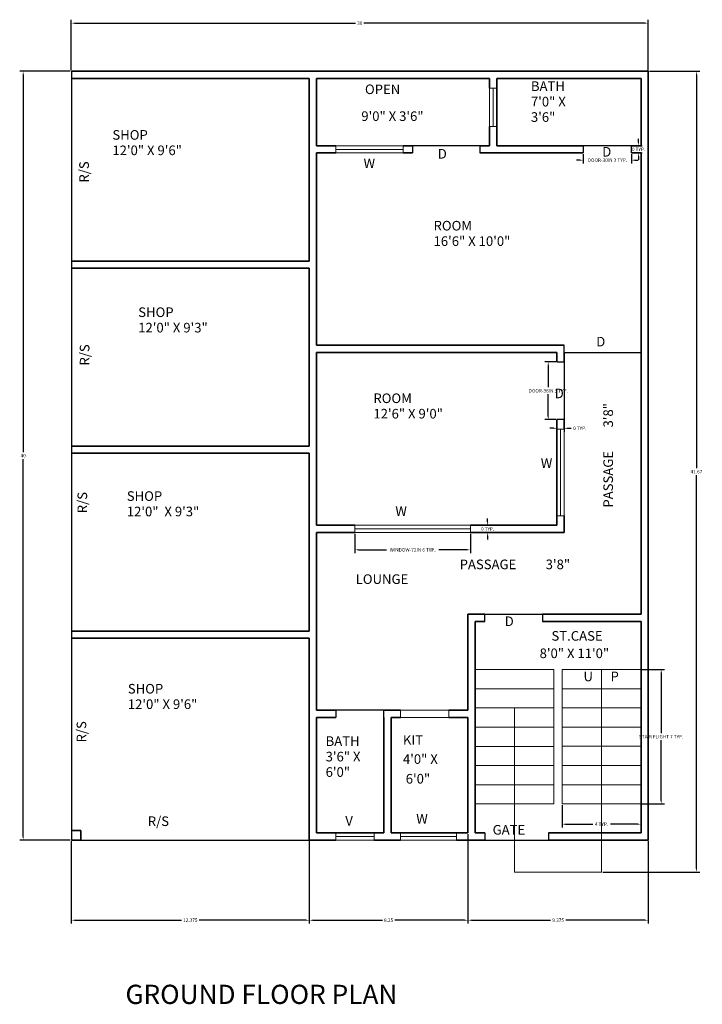
# Model space of a CAD drawing. Units: feet. Extents: x 60.2 to 151.6, y 170.7 to 222.6.
# Tile 1 of 3: x 60.2 to 95.6, y 171.3 to 222.6. Entities that reach past the tile are written whole.
import ezdxf

# ---------------------------------------------------------------- set-up
doc = ezdxf.new("R2010")
doc.units = ezdxf.units.FT
for name, color, linetype, lineweight in [('A-ANNO-DIMS', 7, 'Continuous', 13), ('A-ANNO-TEXT', 7, 'Continuous', 13), ('A-ANNO-TITL', 7, 'Continuous', 25), ('A-AREA-IDEN', 7, 'Continuous', 18), ('A-DOOR', 6, 'Continuous', 25), ('A-FLOR-STRS', 6, 'Continuous', 18), ('A-GLAZ', 240, 'Continuous', 18), ('A-WALL', 175, 'Continuous', 35)]:
    doc.layers.add(name, color=color, linetype=linetype, lineweight=lineweight)
doc.styles.get("Standard").update_dxf_attribs({"font": 'arial.ttf'})
doc.dimstyles.get("Standard").update_dxf_attribs({"dimtxt": 0.18, "dimasz": 0.18, "dimexe": 0.18, "dimexo": 0.0625, "dimgap": 0.09, "dimtad": 0, "dimtih": 1, "dimtoh": 1, "dimdec": 4, "dimzin": 0, "dimdsep": 46, "dimtxsty": 'Standard', "dimcen": 0.09, "dimadec": 0, "dimazin": 0, "dimtfac": 1, "dimtdec": 4, "dimtofl": 0, "dimtmove": 0, "dimatfit": 3, "dimfxl": 1, "dimtolj": 1, "dimtzin": 0, "dimarcsym": 0})

# ---------------------------------------------------------------- blocks, each defined once
blk = doc.blocks.new('DOOR-30IN')
for p, q in [((2.5, 0.375), (0, 0.375)), ((0, 0.375), (0, 0)), ((2.5, 0), (2.5, 0.375))]:
    blk.add_line(p, q)
blk = doc.blocks.new('DOOR-36IN')
for p, q in [((0, 0.375), (3, 0.375)), ((0, 0), (0, 0.375)), ((3, 0.375), (3, 0))]:
    blk.add_line(p, q)
blk = doc.blocks.new('DOOR-42IN')
for p, q in [((3.5, 0.375), (0, 0.375)), ((0, 0.375), (0, 0)), ((3.5, 0.375), (3.5, 0))]:
    blk.add_line(p, q)
blk = doc.blocks.new('WINDOW-24IN')
for p, q in [((0, 2), (0.375, 2)), ((0, 2), (0, 0)), ((0.188, 2), (0.188, 0)), ((0.375, 2), (0.375, 0)), ((0, 0), (0.375, 0))]:
    blk.add_line(p, q)
blk = doc.blocks.new('STAIR-FLIGHT-8-TREADS')
for p, q in [((0, 7), (4.1, 7)), ((4.1, 7), (4.1, 0)), ((0, 6), (4.1, 6)), ((0, 5), (4.1, 5)), ((0, 4), (4.1, 4)), ((0, 3), (4.1, 3)), ((0, 2), (4.1, 2)), ((0, 1), (4.1, 1)), ((0, 0), (4.1, 0))]:
    blk.add_line(p, q)
blk = doc.blocks.new('SHOP-BAY-WALL-12FT-X-9FT3IN')
for p, q in [((0.375, 9.25), (0, 9.25)), ((12.375, 9.25), (0.375, 9.25)), ((0.375, 9.25), (12.375, 9.25)), ((12.375, 9.25), (12.375, 0)), ((0.375, 0), (0, 0)), ((12.375, 0), (0.375, 0))]:
    blk.add_line(p, q)
blk = doc.blocks.new('WINDOW-72IN')
for p, q in [((0, 0.375), (0, 0)), ((6, 0.375), (0, 0.375)), ((0, 0.188), (6, 0.188)), ((6, 0), (0, 0)), ((6, 0), (6, 0.375))]:
    blk.add_line(p, q)
blk = doc.blocks.new('*D14')
at = {"layer": 'A-ANNO-DIMS', "color": 0, "lineweight": -2, "transparency": 16777216}
for p, q in [((89.282, 215.268), (89.102, 215.268)), ((89.462, 215.581), (89.462, 215.088)), ((91.962, 215.581), (91.962, 215.088)), ((92.142, 215.268), (92.322, 215.268))]:
    blk.add_line(p, q, dxfattribs=at)
at = {"layer": 'A-ANNO-DIMS', "color": 0, "transparency": 16777216}
for points in [[(89.282, 215.298), (89.282, 215.238), (89.462, 215.268)], [(92.142, 215.298), (92.142, 215.238), (91.962, 215.268)]]:
    blk.add_solid(points, dxfattribs=at)
at = {"layer": 'Defpoints', "color": 0, "transparency": 16777216}
for p in [(89.462, 215.643), (91.962, 215.643), (91.962, 215.268)]:
    blk.add_point(p, dxfattribs=at)
at = {"layer": 'A-ANNO-DIMS', "color": 0, "transparency": 16777216, "insert": (90.712, 215.268), "char_height": 0.18, "attachment_point": 5}
blk.add_mtext('\\A1;DOOR-30IN 3 TYP.', dxfattribs=at)
blk = doc.blocks.new('*D15')
at = {"layer": 'A-ANNO-DIMS', "color": 0, "lineweight": -2, "transparency": 16777216}
for p, q in [((92.337, 216.198), (92.337, 216.378)), ((92.025, 216.018), (92.517, 216.018)), ((92.025, 215.643), (92.517, 215.643)), ((92.337, 215.463), (92.337, 215.283))]:
    blk.add_line(p, q, dxfattribs=at)
at = {"layer": 'A-ANNO-DIMS', "color": 0, "transparency": 16777216}
for points in [[(92.307, 216.198), (92.367, 216.198), (92.337, 216.018)], [(92.307, 215.463), (92.367, 215.463), (92.337, 215.643)]]:
    blk.add_solid(points, dxfattribs=at)
at = {"layer": 'Defpoints', "color": 0, "transparency": 16777216}
for p in [(91.962, 216.018), (92.337, 216.018), (91.962, 215.643)]:
    blk.add_point(p, dxfattribs=at)
at = {"layer": 'A-ANNO-DIMS', "color": 0, "transparency": 16777216, "insert": (92.337, 215.831), "char_height": 0.18, "attachment_point": 5}
blk.add_mtext('\\A1;0 TYP.', dxfattribs=at)
blk = doc.blocks.new('*D16')
at = {"layer": 'A-ANNO-DIMS', "color": 0, "lineweight": -2, "transparency": 16777216}
for p, q in [((88.025, 204.768), (87.457, 204.768)), ((87.637, 204.588), (87.637, 203.451)), ((87.637, 201.948), (87.637, 203.085)), ((88.025, 201.768), (87.457, 201.768))]:
    blk.add_line(p, q, dxfattribs=at)
at = {"layer": 'A-ANNO-DIMS', "color": 0, "transparency": 16777216}
for points in [[(87.607, 204.588), (87.667, 204.588), (87.637, 204.768)], [(87.607, 201.948), (87.667, 201.948), (87.637, 201.768)]]:
    blk.add_solid(points, dxfattribs=at)
at = {"layer": 'Defpoints', "color": 0, "transparency": 16777216}
for p in [(88.087, 204.768), (87.637, 201.768), (88.087, 201.768)]:
    blk.add_point(p, dxfattribs=at)
at = {"layer": 'A-ANNO-DIMS', "color": 0, "transparency": 16777216, "insert": (87.637, 203.268), "char_height": 0.18, "attachment_point": 5}
blk.add_mtext('\\A1;DOOR-36IN 3 TYP.', dxfattribs=at)
blk = doc.blocks.new('*D17')
at = {"layer": 'A-ANNO-DIMS', "color": 0, "lineweight": -2, "transparency": 16777216}
for p, q in [((88.087, 201.706), (88.087, 201.138)), ((88.462, 201.706), (88.462, 201.138)), ((87.907, 201.318), (87.727, 201.318)), ((88.642, 201.318), (88.822, 201.318))]:
    blk.add_line(p, q, dxfattribs=at)
at = {"layer": 'A-ANNO-DIMS', "color": 0, "transparency": 16777216}
for points in [[(87.907, 201.348), (87.907, 201.288), (88.087, 201.318)], [(88.642, 201.348), (88.642, 201.288), (88.462, 201.318)]]:
    blk.add_solid(points, dxfattribs=at)
at = {"layer": 'Defpoints', "color": 0, "transparency": 16777216}
for p in [(88.087, 201.768), (88.462, 201.768), (88.462, 201.318)]:
    blk.add_point(p, dxfattribs=at)
at = {"layer": 'A-ANNO-DIMS', "color": 0, "transparency": 16777216, "insert": (89.28, 201.318), "char_height": 0.18, "attachment_point": 5}
blk.add_mtext('\\A1;0 TYP.', dxfattribs=at)
blk = doc.blocks.new('*D32')
at = {"layer": 'A-ANNO-DIMS', "color": 0, "lineweight": -2, "transparency": 16777216}
for p, q in [((77.587, 195.831), (77.587, 194.813)), ((83.587, 195.831), (83.587, 194.813)), ((77.767, 194.993), (79.231, 194.993)), ((83.407, 194.993), (81.943, 194.993))]:
    blk.add_line(p, q, dxfattribs=at)
at = {"layer": 'A-ANNO-DIMS', "color": 0, "transparency": 16777216}
for points in [[(77.767, 195.023), (77.767, 194.963), (77.587, 194.993)], [(83.407, 195.023), (83.407, 194.963), (83.587, 194.993)]]:
    blk.add_solid(points, dxfattribs=at)
at = {"layer": 'Defpoints', "color": 0, "transparency": 16777216}
for p in [(77.587, 195.893), (83.587, 195.893), (83.587, 194.993)]:
    blk.add_point(p, dxfattribs=at)
at = {"layer": 'A-ANNO-DIMS', "color": 0, "transparency": 16777216, "insert": (80.587, 194.993), "char_height": 0.18, "attachment_point": 5}
blk.add_mtext('\\A1;WINDOW-72IN 6 TYP.', dxfattribs=at)
blk = doc.blocks.new('*D33')
at = {"layer": 'A-ANNO-DIMS', "color": 0, "lineweight": -2, "transparency": 16777216}
for p, q in [((83.65, 196.268), (84.667, 196.268)), ((84.487, 196.448), (84.487, 196.628)), ((83.65, 195.893), (84.667, 195.893)), ((84.487, 195.713), (84.487, 195.533))]:
    blk.add_line(p, q, dxfattribs=at)
at = {"layer": 'A-ANNO-DIMS', "color": 0, "transparency": 16777216}
for points in [[(84.457, 196.448), (84.517, 196.448), (84.487, 196.268)], [(84.457, 195.713), (84.517, 195.713), (84.487, 195.893)]]:
    blk.add_solid(points, dxfattribs=at)
at = {"layer": 'Defpoints', "color": 0, "transparency": 16777216}
for p in [(83.587, 196.268), (84.487, 196.268), (83.587, 195.893)]:
    blk.add_point(p, dxfattribs=at)
at = {"layer": 'A-ANNO-DIMS', "color": 0, "transparency": 16777216, "insert": (84.487, 196.081), "char_height": 0.18, "attachment_point": 5}
blk.add_mtext('\\A1;0 TYP.', dxfattribs=at)
blk = doc.blocks.new('*D34')
at = {"layer": 'A-ANNO-DIMS', "color": 0, "lineweight": -2, "transparency": 16777216}
for p, q in [((92.525, 188.768), (93.692, 188.768)), ((93.512, 188.588), (93.512, 185.451)), ((93.512, 181.948), (93.512, 185.085)), ((92.525, 181.768), (93.692, 181.768))]:
    blk.add_line(p, q, dxfattribs=at)
at = {"layer": 'A-ANNO-DIMS', "color": 0, "transparency": 16777216}
for points in [[(93.482, 188.588), (93.542, 188.588), (93.512, 188.768)], [(93.482, 181.948), (93.542, 181.948), (93.512, 181.768)]]:
    blk.add_solid(points, dxfattribs=at)
at = {"layer": 'Defpoints', "color": 0, "transparency": 16777216}
for p in [(92.462, 188.768), (92.462, 181.768), (93.512, 181.768)]:
    blk.add_point(p, dxfattribs=at)
at = {"layer": 'A-ANNO-DIMS', "color": 0, "transparency": 16777216, "insert": (93.512, 185.268), "char_height": 0.18, "attachment_point": 5}
blk.add_mtext('\\A1;STAIR FLIGHT 7 TYP.', dxfattribs=at)
blk = doc.blocks.new('*D35')
at = {"layer": 'A-ANNO-DIMS', "color": 0, "lineweight": -2, "transparency": 16777216}
for p, q in [((88.362, 181.706), (88.362, 180.538)), ((92.462, 181.706), (92.462, 180.538)), ((88.542, 180.718), (89.95, 180.718)), ((92.282, 180.718), (90.874, 180.718))]:
    blk.add_line(p, q, dxfattribs=at)
at = {"layer": 'A-ANNO-DIMS', "color": 0, "transparency": 16777216}
for points in [[(88.542, 180.748), (88.542, 180.688), (88.362, 180.718)], [(92.282, 180.748), (92.282, 180.688), (92.462, 180.718)]]:
    blk.add_solid(points, dxfattribs=at)
at = {"layer": 'Defpoints', "color": 0, "transparency": 16777216}
for p in [(88.362, 181.768), (92.462, 181.768), (88.362, 180.718)]:
    blk.add_point(p, dxfattribs=at)
at = {"layer": 'A-ANNO-DIMS', "color": 0, "transparency": 16777216, "insert": (90.412, 180.718), "char_height": 0.18, "attachment_point": 5}
blk.add_mtext('\\A1;4 TYP.', dxfattribs=at)
blk = doc.blocks.new('*D38')
at = {"layer": 'A-ANNO-DIMS', "color": 0, "lineweight": -2, "transparency": 16777216}
for p, q in [((62.837, 219.956), (62.837, 222.578)), ((63.017, 222.398), (77.619, 222.398)), ((92.657, 222.398), (78.056, 222.398)), ((92.837, 219.956), (92.837, 222.578))]:
    blk.add_line(p, q, dxfattribs=at)
at = {"layer": 'A-ANNO-DIMS', "color": 0, "transparency": 16777216}
for points in [[(63.017, 222.428), (63.017, 222.368), (62.837, 222.398)], [(92.657, 222.428), (92.657, 222.368), (92.837, 222.398)]]:
    blk.add_solid(points, dxfattribs=at)
at = {"layer": 'Defpoints', "color": 0, "transparency": 16777216}
for p in [(92.837, 222.398), (62.837, 219.893), (92.837, 219.893)]:
    blk.add_point(p, dxfattribs=at)
at = {"layer": 'A-ANNO-DIMS', "color": 0, "transparency": 16777216, "insert": (77.837, 222.398), "char_height": 0.18, "attachment_point": 5}
blk.add_mtext('\\A1;30', dxfattribs=at)
blk = doc.blocks.new('*D39')
at = {"layer": 'A-ANNO-DIMS', "color": 0, "lineweight": -2, "transparency": 16777216}
for p, q in [((92.9, 219.893), (95.522, 219.893)), ((95.342, 219.713), (95.342, 199.242)), ((95.342, 178.406), (95.342, 198.878)), ((90.475, 178.226), (95.522, 178.226))]:
    blk.add_line(p, q, dxfattribs=at)
at = {"layer": 'A-ANNO-DIMS', "color": 0, "transparency": 16777216}
for points in [[(95.312, 219.713), (95.372, 219.713), (95.342, 219.893)], [(95.312, 178.406), (95.372, 178.406), (95.342, 178.226)]]:
    blk.add_solid(points, dxfattribs=at)
at = {"layer": 'Defpoints', "color": 0, "transparency": 16777216}
for p in [(92.837, 219.893), (95.342, 219.893), (90.412, 178.226)]:
    blk.add_point(p, dxfattribs=at)
at = {"layer": 'A-ANNO-DIMS', "color": 0, "transparency": 16777216, "insert": (95.342, 199.06), "char_height": 0.18, "attachment_point": 5}
blk.add_mtext('\\A1;41.67', dxfattribs=at)
blk = doc.blocks.new('*D40')
at = {"layer": 'A-ANNO-DIMS', "color": 0, "lineweight": -2, "transparency": 16777216}
for p, q in [((62.775, 219.893), (60.152, 219.893)), ((60.332, 219.713), (60.332, 200.075)), ((60.332, 180.073), (60.332, 199.711)), ((62.775, 179.893), (60.152, 179.893))]:
    blk.add_line(p, q, dxfattribs=at)
at = {"layer": 'A-ANNO-DIMS', "color": 0, "transparency": 16777216}
for points in [[(60.302, 219.713), (60.362, 219.713), (60.332, 219.893)], [(60.302, 180.073), (60.362, 180.073), (60.332, 179.893)]]:
    blk.add_solid(points, dxfattribs=at)
at = {"layer": 'Defpoints', "color": 0, "transparency": 16777216}
for p in [(60.332, 219.893), (62.837, 219.893), (62.837, 179.893)]:
    blk.add_point(p, dxfattribs=at)
at = {"layer": 'A-ANNO-DIMS', "color": 0, "transparency": 16777216, "insert": (60.332, 199.893), "char_height": 0.18, "attachment_point": 5}
blk.add_mtext('\\A1;40', dxfattribs=at)
blk = doc.blocks.new('*D41')
at = {"layer": 'A-ANNO-DIMS', "color": 0, "lineweight": -2, "transparency": 16777216}
for p, q in [((62.837, 179.831), (62.837, 175.541)), ((75.212, 179.831), (75.212, 175.541)), ((63.017, 175.721), (68.569, 175.721)), ((75.032, 175.721), (69.481, 175.721))]:
    blk.add_line(p, q, dxfattribs=at)
at = {"layer": 'A-ANNO-DIMS', "color": 0, "transparency": 16777216}
for points in [[(63.017, 175.751), (63.017, 175.691), (62.837, 175.721)], [(75.032, 175.751), (75.032, 175.691), (75.212, 175.721)]]:
    blk.add_solid(points, dxfattribs=at)
at = {"layer": 'Defpoints', "color": 0, "transparency": 16777216}
for p in [(62.837, 179.893), (75.212, 179.893), (75.212, 175.721)]:
    blk.add_point(p, dxfattribs=at)
at = {"layer": 'A-ANNO-DIMS', "color": 0, "transparency": 16777216, "insert": (69.025, 175.721), "char_height": 0.18, "attachment_point": 5}
blk.add_mtext('\\A1;12.375', dxfattribs=at)
blk = doc.blocks.new('*D42')
at = {"layer": 'A-ANNO-DIMS', "color": 0, "lineweight": -2, "transparency": 16777216}
for p, q in [((75.212, 179.831), (75.212, 175.541)), ((83.462, 180.206), (83.462, 175.541)), ((75.392, 175.721), (79.013, 175.721)), ((83.282, 175.721), (79.662, 175.721))]:
    blk.add_line(p, q, dxfattribs=at)
at = {"layer": 'A-ANNO-DIMS', "color": 0, "transparency": 16777216}
for points in [[(75.392, 175.751), (75.392, 175.691), (75.212, 175.721)], [(83.282, 175.751), (83.282, 175.691), (83.462, 175.721)]]:
    blk.add_solid(points, dxfattribs=at)
at = {"layer": 'Defpoints', "color": 0, "transparency": 16777216}
for p in [(75.212, 179.893), (83.462, 180.268), (83.462, 175.721)]:
    blk.add_point(p, dxfattribs=at)
at = {"layer": 'A-ANNO-DIMS', "color": 0, "transparency": 16777216, "insert": (79.337, 175.721), "char_height": 0.18, "attachment_point": 5}
blk.add_mtext('\\A1;8.25', dxfattribs=at)
blk = doc.blocks.new('*D43')
at = {"layer": 'A-ANNO-DIMS', "color": 0, "lineweight": -2, "transparency": 16777216}
for p, q in [((83.462, 180.206), (83.462, 175.541)), ((92.837, 179.831), (92.837, 175.541)), ((83.642, 175.721), (87.755, 175.721)), ((92.657, 175.721), (88.544, 175.721))]:
    blk.add_line(p, q, dxfattribs=at)
at = {"layer": 'A-ANNO-DIMS', "color": 0, "transparency": 16777216}
for points in [[(83.642, 175.751), (83.642, 175.691), (83.462, 175.721)], [(92.657, 175.751), (92.657, 175.691), (92.837, 175.721)]]:
    blk.add_solid(points, dxfattribs=at)
at = {"layer": 'Defpoints', "color": 0, "transparency": 16777216}
for p in [(83.462, 180.268), (92.837, 179.893), (92.837, 175.721)]:
    blk.add_point(p, dxfattribs=at)
at = {"layer": 'A-ANNO-DIMS', "color": 0, "transparency": 16777216, "insert": (88.15, 175.721), "char_height": 0.18, "attachment_point": 5}
blk.add_mtext('\\A1;9.375', dxfattribs=at)

msp = doc.modelspace()

# ---------------------------------------------------------------- linework, layer by layer
at = {"layer": 'A-DOOR'}
for p, q in [((88.4623, 205.2682), (88.4623, 205.6432)), ((88.4623, 205.2682), (92.4623, 205.2682)), ((84.3373, 180.2682), (84.3373, 179.8932)), ((87.6498, 180.2682), (87.6498, 179.8932))]:
    msp.add_line(p, q, dxfattribs=at)
for points in [[(62.8373, 219.8932), (62.8373, 179.8932)], [(62.8373, 179.8932), (75.2123, 179.8932)], [(84.3373, 179.8932), (87.6498, 179.8932)]]:
    msp.add_lwpolyline(points, dxfattribs=at)
at = {"layer": 'A-FLOR-STRS'}
for p, q in [((90.4123, 178.2264), (90.4123, 188.7682)), ((85.8873, 186.7682), (85.8873, 178.2264)), ((85.8873, 178.2264), (90.4123, 178.2264))]:
    msp.add_line(p, q, dxfattribs=at)
at = {"layer": 'A-GLAZ'}
for p, q in [((76.5873, 216.0182), (76.5873, 215.6432)), ((80.0873, 216.0182), (76.5873, 216.0182)), ((76.5873, 215.8307), (80.0873, 215.8307)), ((80.0873, 215.6432), (80.0873, 216.0182)), ((80.0873, 215.6432), (76.5873, 215.6432)), ((88.0873, 200.7682), (88.0873, 201.2682)), ((88.0873, 201.2682), (88.4623, 201.2682)), ((88.2748, 201.2682), (88.2748, 196.7682)), ((88.4623, 201.2682), (88.4623, 196.7682)), ((88.0873, 196.7682), (88.0873, 200.7682)), ((88.0873, 196.7682), (88.4623, 196.7682)), ((77.5873, 195.8932), (81.5873, 195.8932)), ((81.5873, 195.8932), (82.5873, 195.8932)), ((82.5873, 195.8932), (83.5873, 195.8932)), ((79.9623, 186.2682), (79.9623, 186.6432)), ((82.4623, 186.6432), (79.9623, 186.6432)), ((82.4623, 186.6432), (82.4623, 186.2682)), ((82.4623, 186.2682), (79.9623, 186.2682)), ((76.5873, 180.2682), (76.5873, 179.8932)), ((76.5873, 180.2682), (78.5873, 180.2682)), ((76.5873, 180.0807), (78.5873, 180.0807)), ((78.5873, 180.2682), (78.5873, 179.8932)), ((79.9623, 180.2682), (79.9623, 179.8932)), ((79.9623, 180.2682), (82.8623, 180.2682)), ((79.9623, 180.0807), (82.8623, 180.0807)), ((82.8623, 180.2682), (82.8623, 179.8932))]:
    msp.add_line(p, q, dxfattribs=at)
for points in [[(76.5873, 179.8932), (78.5873, 179.8932)], [(79.9623, 179.8932), (82.8623, 179.8932)]]:
    msp.add_lwpolyline(points, dxfattribs=at)
at = {"layer": 'A-WALL'}
for p, q in [((63.2123, 219.5182), (62.8373, 219.5182)), ((63.2123, 219.5182), (75.2123, 219.5182)), ((75.2123, 219.5182), (75.2123, 210.0182)), ((75.5873, 219.5182), (75.5873, 216.0182)), ((75.5873, 219.5182), (84.5873, 219.5182)), ((84.5873, 219.5182), (84.5873, 219.0182)), ((84.5873, 219.5182), (84.5873, 219.0182)), ((84.9623, 219.5182), (84.9623, 216.0182)), ((84.9623, 219.5182), (84.9623, 219.0182)), ((84.5873, 216.0182), (84.5873, 217.0182)), ((84.5873, 217.0182), (84.5873, 216.0182)), ((84.9623, 217.0182), (84.9623, 216.0182)), ((75.5873, 216.0182), (76.5873, 216.0182)), ((76.5873, 216.0182), (75.5873, 216.0182)), ((80.0873, 216.0182), (80.5873, 216.0182)), ((80.5873, 216.0182), (80.0873, 216.0182)), ((84.5873, 216.0182), (84.0873, 216.0182)), ((84.5873, 216.0182), (84.0873, 216.0182)), ((84.9623, 216.0182), (89.4623, 216.0182)), ((84.9623, 216.0182), (88.4623, 216.0182)), ((88.4623, 216.0182), (89.4623, 216.0182)), ((91.9623, 216.0182), (92.4623, 216.0182)), ((92.4623, 216.0182), (91.9623, 216.0182)), ((75.5873, 215.6432), (75.5873, 205.6432)), ((75.5873, 215.6432), (75.5873, 210.0182)), ((76.5873, 215.6432), (75.5873, 215.6432)), ((80.5873, 215.6432), (80.0873, 215.6432)), ((80.5873, 215.6432), (80.0873, 215.6432)), ((84.0873, 215.6432), (84.9623, 215.6432)), ((84.9623, 215.6432), (89.4623, 215.6432)), ((91.9623, 215.6432), (92.4623, 215.6432)), ((63.2123, 210.0182), (62.8373, 210.0182)), ((75.2123, 210.0182), (63.2123, 210.0182)), ((75.5873, 209.6432), (75.5873, 205.6432)), ((75.5873, 205.6432), (88.4623, 205.6432)), ((75.5873, 205.2682), (88.0873, 205.2682)), ((75.5873, 205.2682), (88.0873, 205.2682)), ((75.5873, 205.2682), (75.5873, 200.3932)), ((88.0873, 205.2682), (88.0873, 204.7682)), ((88.0873, 205.2682), (88.0873, 204.7682)), ((88.4623, 205.2682), (88.4623, 204.7682)), ((88.0873, 201.2682), (88.0873, 201.7682)), ((88.0873, 201.7682), (88.0873, 196.2682)), ((88.4623, 201.7682), (88.4623, 201.2682)), ((75.5873, 200.3932), (75.5873, 200.0182)), ((75.5873, 200.0182), (75.5873, 196.2682)), ((88.0873, 196.2682), (88.0873, 196.7682)), ((88.0873, 196.2682), (88.0873, 196.7682)), ((88.4623, 196.7682), (88.4623, 196.2682)), ((75.5873, 196.2682), (77.5873, 196.2682)), ((77.5873, 196.2682), (75.5873, 196.2682)), ((88.0873, 196.2682), (83.5873, 196.2682)), ((88.4623, 196.2682), (88.4623, 195.8932)), ((75.5873, 195.8932), (75.5873, 190.7682)), ((77.5873, 195.8932), (75.5873, 195.8932)), ((88.0873, 195.8932), (83.5873, 195.8932)), ((88.4623, 195.8932), (88.0873, 195.8932)), ((83.8373, 191.6432), (83.4623, 191.6432)), ((83.4623, 191.6432), (83.4623, 191.2682)), ((83.8373, 191.6432), (84.3373, 191.6432)), ((87.8373, 191.6432), (87.3373, 191.6432)), ((87.3373, 191.6432), (91.8373, 191.6432)), ((92.4623, 191.6432), (87.8373, 191.6432)), ((91.8373, 191.6432), (92.4623, 191.6432)), ((83.4623, 186.6432), (83.4623, 191.2682)), ((83.8373, 180.2682), (83.8373, 191.2682)), ((83.8373, 191.2682), (84.3373, 191.2682)), ((83.8373, 191.2682), (84.3373, 191.2682)), ((87.3373, 191.2682), (91.8373, 191.2682)), ((91.8373, 191.2682), (92.4623, 191.2682)), ((75.5873, 190.7682), (75.5873, 190.3932)), ((63.2123, 190.3932), (62.8373, 190.3932)), ((75.2123, 190.3932), (63.2123, 190.3932)), ((63.2123, 190.3932), (75.2123, 190.3932)), ((75.2123, 190.3932), (75.2123, 179.8932)), ((75.5873, 190.3932), (75.5873, 186.6432)), ((75.5873, 186.6432), (76.5873, 186.6432)), ((76.5873, 186.6432), (75.5873, 186.6432)), ((79.0873, 186.6432), (79.4623, 186.6432)), ((79.9623, 186.6432), (79.4623, 186.6432)), ((83.4623, 186.6432), (82.4623, 186.6432)), ((82.9623, 186.6432), (82.4623, 186.6432)), ((83.4623, 186.6432), (82.9623, 186.6432)), ((76.5873, 186.2682), (75.5873, 186.2682)), ((75.5873, 186.2682), (75.5873, 180.2682)), ((79.0873, 180.2682), (79.0873, 186.2682)), ((79.4623, 180.2682), (79.4623, 186.2682)), ((79.4623, 186.2682), (79.9623, 186.2682)), ((79.9623, 186.2682), (79.4623, 186.2682)), ((83.4623, 186.2682), (82.4623, 186.2682)), ((83.4623, 180.2682), (83.4623, 186.2682)), ((83.4623, 180.2682), (83.4623, 186.2682)), ((83.8373, 180.2682), (83.8373, 186.2682)), ((63.3373, 180.3932), (62.8373, 180.3932)), ((63.3373, 179.8932), (63.3373, 180.3932)), ((62.8373, 179.8932), (63.3373, 179.8932)), ((75.5873, 180.2682), (76.5873, 180.2682)), ((75.5873, 180.2682), (76.5873, 180.2682)), ((79.0873, 180.2682), (78.5873, 180.2682)), ((78.5873, 180.2682), (79.0873, 180.2682)), ((79.4623, 180.2682), (79.9623, 180.2682)), ((79.4623, 180.2682), (79.9623, 180.2682)), ((83.4623, 180.2682), (82.8623, 180.2682)), ((82.8623, 180.2682), (83.4623, 180.2682)), ((83.8373, 180.2682), (84.3373, 180.2682)), ((88.1498, 180.2682), (87.6498, 180.2682)), ((92.4623, 180.2682), (88.1498, 180.2682))]:
    msp.add_line(p, q, dxfattribs=at)
for points in [[(87.6498, 179.8932), (92.8373, 179.8932), (92.8373, 219.8932), (62.8373, 219.8932)], [(75.2123, 219.5182), (63.2123, 219.5182)], [(84.5873, 219.5182), (75.5873, 219.5182)], [(92.4623, 216.0182), (92.4623, 219.5182), (84.9623, 219.5182)], [(92.4623, 191.6432), (92.4623, 215.6432)], [(87.6498, 180.2682), (92.4623, 180.2682), (92.4623, 191.2682)], [(75.2123, 179.8932), (76.5873, 179.8932)], [(75.5873, 180.2682), (79.0873, 180.2682)], [(78.5873, 179.8932), (79.9623, 179.8932)], [(79.4623, 180.2682), (83.4623, 180.2682)], [(82.8623, 179.8932), (84.3373, 179.8932)], [(83.8373, 180.2682), (84.3373, 180.2682)]]:
    msp.add_lwpolyline(points, dxfattribs=at)

# ---------------------------------------------------------------- block references
at = {"layer": 'A-DOOR'}
for name, p in [('DOOR-42IN', (80.587, 215.643)), ('DOOR-30IN', (89.462, 215.643)), ('DOOR-36IN', (84.337, 191.268)), ('DOOR-30IN', (76.587, 186.268))]:
    msp.add_blockref(name, p, dxfattribs=at)
at = {"layer": 'A-DOOR', "rotation": 269.9999999999999}
msp.add_blockref('DOOR-36IN', (88.0871, 204.7685), dxfattribs=at)
at = {"layer": 'A-FLOR-STRS'}
msp.add_blockref('STAIR-FLIGHT-8-TREADS', (83.837, 181.768), dxfattribs=at)
at = {"layer": 'A-FLOR-STRS', "rotation": 180}
msp.add_blockref('STAIR-FLIGHT-8-TREADS', (92.4625, 188.7684), dxfattribs=at)
at = {"layer": 'A-GLAZ'}
for name, p in [('WINDOW-24IN', (84.587, 217.018)), ('WINDOW-72IN', (77.587, 195.893))]:
    msp.add_blockref(name, p, dxfattribs=at)
at = {"layer": 'A-WALL'}
for p in [(62.837, 200.393), (62.837, 190.768)]:
    msp.add_blockref('SHOP-BAY-WALL-12FT-X-9FT3IN', p, dxfattribs=at)

# ---------------------------------------------------------------- texts
at = {"layer": 'A-ANNO-DIMS'}
for s, p in [('7\'0" X', (86.7368, 218.0655)), ('9\'0" X 3\'6"', (77.9166, 217.3088)), ('3\'6"', (86.7368, 217.2623)), ('12\'0" X 9\'6"', (64.9716, 215.5299)), ('16\'6" X 10\'0"', (81.6736, 210.8062)), ('12\'0" X 9\'3"', (66.3156, 206.3046)), ('12\'6" X 9\'0"', (78.5449, 201.8268)), ('12\'0"  X 9\'3"', (65.7221, 196.7377)), ('8\'0" X 11\'0"', (87.1894, 189.3586)), ('12\'0" X 9\'6"', (65.7757, 186.7114)), ('3\'6" X', (76.0609, 183.9841)), ('4\'0" X', (80.0809, 183.8552)), ('6\'0"', (76.0609, 183.1809)), ('6\'0"', (80.2272, 182.832))]:
    msp.add_text(s, height=0.5, dxfattribs=at).set_placement(p)
at = {"layer": 'A-ANNO-TEXT'}
for s, p in [('D', (81.8958, 215.3501)), ('D', (90.4471, 215.4551)), ('W', (78.0337, 214.8531)), ('D', (90.1352, 205.5758)), ('D', (87.9747, 202.8813)), ('W', (87.2502, 199.252)), ('W', (79.6882, 196.7573)), ('D', (85.3753, 191.0249)), ('U', (89.4714, 188.1567)), ('P', (90.878, 188.1577)), ('R/S', (66.8125, 180.6218)), ('V', (77.0856, 180.6423)), ('W', (80.7745, 180.7447)), ('GATE', (84.7458, 180.1742))]:
    msp.add_text(s, height=0.5, dxfattribs=at).set_placement(p)
for p in [(63.7493, 214.1004), (63.7781, 204.5808), (63.658, 196.8949), (63.612, 184.9696)]:
    msp.add_text('R/S', height=0.5, rotation=90, dxfattribs=at).set_placement(p)
at = {"layer": 'A-ANNO-TITL'}
msp.add_text('GROUND FLOOR PLAN', height=1, dxfattribs=at).set_placement((65.6506, 171.3626))
at = {"layer": 'A-AREA-IDEN'}
for s, p in [('BATH', (86.7368, 218.8687)), ('OPEN', (78.1073, 218.7051)), ('SHOP', (64.9716, 216.3331)), ('ROOM', (81.6736, 211.6094)), ('SHOP', (66.3156, 207.1078)), ('ROOM', (78.5449, 202.63)), ('SHOP', (65.7221, 197.5409)), ('PASSAGE          3\'8"', (83.0301, 193.9861)), ('LOUNGE', (77.6249, 193.2182)), ('ST.CASE', (87.8038, 190.2648)), ('SHOP', (65.7757, 187.5146)), ('BATH', (76.0609, 184.7873)), ('KIT', (80.0809, 184.8492))]:
    msp.add_text(s, height=0.5, dxfattribs=at).set_placement(p)
msp.add_text('PASSAGE        3\'8"', height=0.5, rotation=90, dxfattribs=at).set_placement((91.0053, 197.1911))

# ---------------------------------------------------------------- dimensions: what is measured, and where the dimension line sits
at = {"layer": 'A-ANNO-DIMS'}
for base, p1, p2, override, picture, middle in [((92.8373, 222.3982), (62.8373, 219.8932), (92.8373, 219.8932), {"dimdec": 0, "dimlfac": 1, "dimrnd": 0, "dimzin": 0, "dimdsep": 46, "dimlunit": 2}, '*D38', (77.8373, 222.3982)), ((75.2123, 175.7214), (62.8373, 179.8932), (75.2123, 179.8932), {"dimdec": 3, "dimlfac": 1, "dimrnd": 0, "dimzin": 0, "dimdsep": 46, "dimlunit": 2}, '*D41', (69.0248, 175.7214)), ((83.4623, 175.7214), (75.2123, 179.8932), (83.4623, 180.2682), {"dimdec": 2, "dimlfac": 1, "dimrnd": 0, "dimzin": 0, "dimdsep": 46, "dimlunit": 2}, '*D42', (79.3373, 175.7214)), ((92.8373, 175.7214), (83.4623, 180.2682), (92.8373, 179.8932), {"dimdec": 3, "dimlfac": 1, "dimrnd": 0, "dimzin": 0, "dimdsep": 46, "dimlunit": 2}, '*D43', (88.1498, 175.7214))]:
    dim = msp.add_linear_dim(base=base, p1=p1, p2=p2, dimstyle='Standard', override=override, dxfattribs=at)
    dim.commit()
    dim.dimension.update_dxf_attribs({"geometry": picture, "text_midpoint": middle})
for base, p1, p2, override, picture, middle in [((60.3323, 219.8932), (62.8373, 179.8932), (62.8373, 219.8932), {"dimdec": 0, "dimlfac": 1, "dimrnd": 0, "dimzin": 0, "dimdsep": 46, "dimlunit": 2}, '*D40', (60.3323, 199.8932)), ((95.3423, 219.8932), (90.4123, 178.2264), (92.8373, 219.8932), {"dimdec": 2, "dimlfac": 1, "dimrnd": 0, "dimzin": 0, "dimdsep": 46, "dimlunit": 2}, '*D39', (95.3423, 199.0598))]:
    dim = msp.add_linear_dim(base=base, p1=p1, p2=p2, angle=90, dimstyle='Standard', override=override, dxfattribs=at)
    dim.commit()
    dim.dimension.update_dxf_attribs({"geometry": picture, "text_midpoint": middle})
for base, p1, p2, angle, text, picture, middle in [((92.3373, 216.0182), (91.9623, 215.6432), (91.9623, 216.0182), 90, '<> TYP.', '*D15', (92.3373, 215.8307)), ((87.6373, 201.7682), (88.0873, 204.7682), (88.0873, 201.7682), 270, 'DOOR-36IN <> TYP.', '*D16', (87.6373, 203.2682)), ((84.4873, 196.2682), (83.5873, 195.8932), (83.5873, 196.2682), 90, '<> TYP.', '*D33', (84.4873, 196.0807)), ((93.5123, 181.7682), (92.4623, 188.7682), (92.4623, 181.7682), 270, 'STAIR FLIGHT <> TYP.', '*D34', (93.5123, 185.2682)), ((88.3623, 180.7182), (92.4623, 181.7682), (88.3623, 181.7682), 180, '<> TYP.', '*D35', (90.4123, 180.7182))]:
    dim = msp.add_linear_dim(base=base, p1=p1, p2=p2, angle=angle, text=text, dimstyle='Standard', override={"dimdec": 0, "dimlfac": 1, "dimrnd": 0, "dimzin": 0, "dimdsep": 46, "dimlunit": 2}, dxfattribs=at)
    dim.commit()
    dim.dimension.update_dxf_attribs({"geometry": picture, "text_midpoint": middle})
for base, p1, p2, text, picture, middle in [((91.962252404, 215.2682003807), (89.462252404, 215.6432003807), (91.962252404, 215.6432003807), 'DOOR-30IN <> TYP.', '*D14', (90.712252404, 215.2682003807)), ((88.4623, 201.3182), (88.0873, 201.7682), (88.4623, 201.7682), '<> TYP.', '*D17', (89.2804, 201.3182)), ((83.5873, 194.9932), (77.5873, 195.8932), (83.5873, 195.8932), 'WINDOW-72IN <> TYP.', '*D32', (80.5873, 194.9932))]:
    dim = msp.add_linear_dim(base=base, p1=p1, p2=p2, text=text, dimstyle='Standard', override={"dimdec": 0, "dimlfac": 1, "dimrnd": 0, "dimzin": 0, "dimdsep": 46, "dimlunit": 2}, dxfattribs=at)
    dim.commit()
    dim.dimension.update_dxf_attribs({"geometry": picture, "text_midpoint": middle})

doc.saveas('drawing.dxf')
